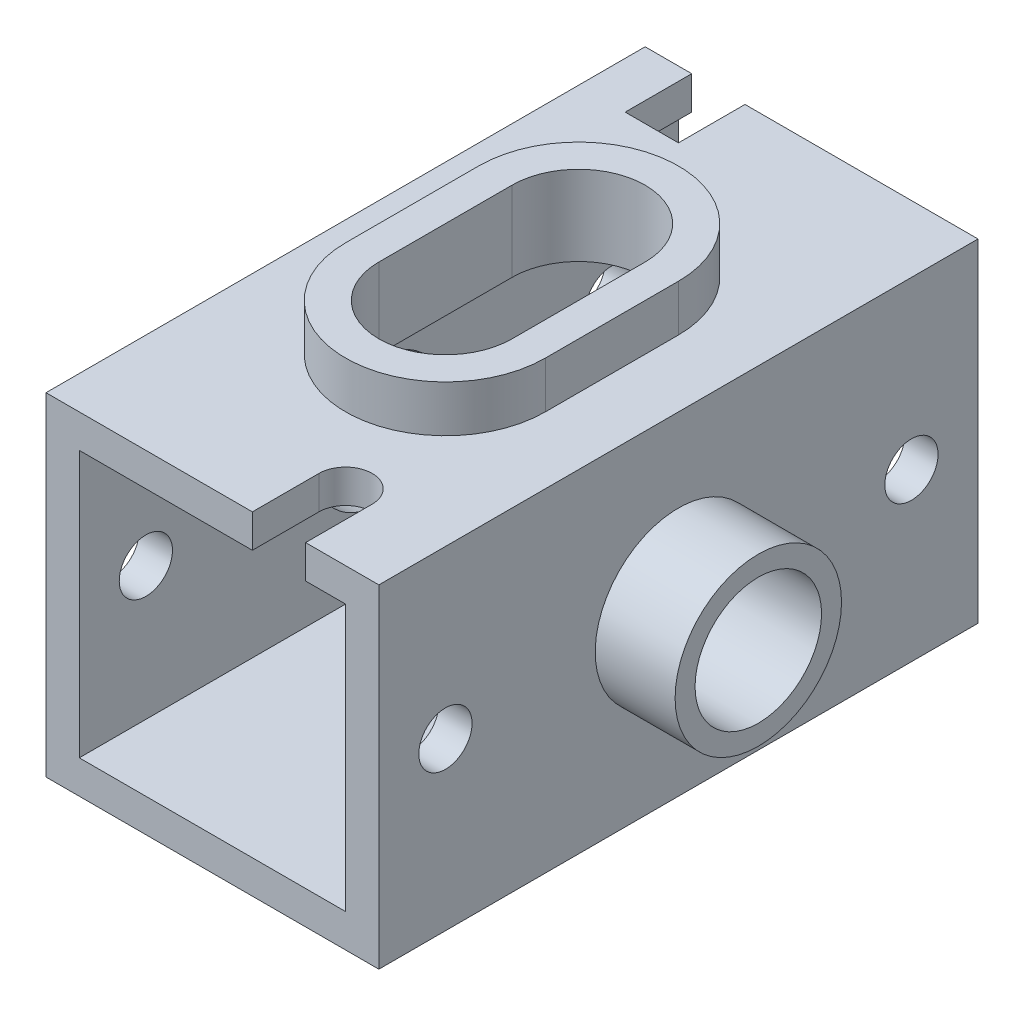
ISO-10303-21;
HEADER;
FILE_DESCRIPTION(('STEP AP214'),'2;1');
FILE_NAME('part.step','',(''),(''),'','','');
FILE_SCHEMA(('AUTOMOTIVE_DESIGN { 1 0 10303 214 1 1 1 1 }'));
ENDSEC;
DATA;
#1=APPLICATION_CONTEXT('core data for automotive mechanical design processes');
#2=APPLICATION_PROTOCOL_DEFINITION('international standard','automotive_design',2000,#1);
#3=PRODUCT_CONTEXT('',#1,'mechanical');
#4=PRODUCT('Part','Part','',(#3));
#5=PRODUCT_RELATED_PRODUCT_CATEGORY('part','',(#4));
#6=PRODUCT_DEFINITION_FORMATION('','',#4);
#7=PRODUCT_DEFINITION_CONTEXT('part definition',#1,'design');
#8=PRODUCT_DEFINITION('design','',#6,#7);
#9=PRODUCT_DEFINITION_SHAPE('','',#8);
#10=(LENGTH_UNIT() NAMED_UNIT(*) SI_UNIT(.MILLI.,.METRE.));
#11=(NAMED_UNIT(*) PLANE_ANGLE_UNIT() SI_UNIT($,.RADIAN.));
#12=(NAMED_UNIT(*) SI_UNIT($,.STERADIAN.) SOLID_ANGLE_UNIT());
#13=UNCERTAINTY_MEASURE_WITH_UNIT(LENGTH_MEASURE(1.E-05),#10,'distance_accuracy_value','');
#14=(GEOMETRIC_REPRESENTATION_CONTEXT(3) GLOBAL_UNCERTAINTY_ASSIGNED_CONTEXT((#13)) GLOBAL_UNIT_ASSIGNED_CONTEXT((#10,
#11,#12)) REPRESENTATION_CONTEXT('',''));
#15=CARTESIAN_POINT('',(0.,0.,0.));
#16=DIRECTION('',(0.,0.,1.));
#17=DIRECTION('',(1.,0.,0.));
#18=AXIS2_PLACEMENT_3D('',#15,#16,#17);
#19=CARTESIAN_POINT('',(-25.,25.,90.));
#20=DIRECTION('',(0.,-1.,0.));
#21=DIRECTION('',(0.,0.,-1.));
#22=AXIS2_PLACEMENT_3D('',#19,#20,#21);
#23=PLANE('',#22);
#24=DIRECTION('',(-1.,0.,0.));
#25=VECTOR('',#24,1.);
#26=CARTESIAN_POINT('',(-25.,25.,90.));
#27=LINE('',#26,#25);
#28=CARTESIAN_POINT('',(5.99999999999999,25.,90.));
#29=VERTEX_POINT('',#28);
#30=CARTESIAN_POINT('',(-25.,25.,90.));
#31=VERTEX_POINT('',#30);
#32=EDGE_CURVE('E400',#29,#31,#27,.T.);
#33=ORIENTED_EDGE('',*,*,#32,.F.);
#34=DIRECTION('',(0.,0.,1.));
#35=VECTOR('',#34,1.);
#36=CARTESIAN_POINT('',(5.99999999999999,25.,80.));
#37=LINE('',#36,#35);
#38=CARTESIAN_POINT('',(5.99999999999999,25.,80.));
#39=VERTEX_POINT('',#38);
#40=EDGE_CURVE('E314',#39,#29,#37,.T.);
#41=ORIENTED_EDGE('',*,*,#40,.F.);
#42=CARTESIAN_POINT('',(9.99999999999999,25.,80.));
#43=DIRECTION('',(0.,1.,0.));
#44=DIRECTION('',(0.,0.,1.));
#45=AXIS2_PLACEMENT_3D('',#42,#43,#44);
#46=CIRCLE('',#45,4.);
#47=CARTESIAN_POINT('',(14.,25.,80.));
#48=VERTEX_POINT('',#47);
#49=EDGE_CURVE('E323',#48,#39,#46,.T.);
#50=ORIENTED_EDGE('',*,*,#49,.F.);
#51=DIRECTION('',(0.,0.,-1.));
#52=VECTOR('',#51,1.);
#53=CARTESIAN_POINT('',(14.,25.,90.));
#54=LINE('',#53,#52);
#55=CARTESIAN_POINT('',(14.,25.,90.));
#56=VERTEX_POINT('',#55);
#57=EDGE_CURVE('E325',#56,#48,#54,.T.);
#58=ORIENTED_EDGE('',*,*,#57,.F.);
#59=CARTESIAN_POINT('',(25.,25.,90.));
#60=VERTEX_POINT('',#59);
#61=EDGE_CURVE('E405',#60,#56,#27,.T.);
#62=ORIENTED_EDGE('',*,*,#61,.F.);
#63=DIRECTION('',(0.,0.,-1.));
#64=VECTOR('',#63,1.);
#65=CARTESIAN_POINT('',(25.,25.,90.));
#66=LINE('',#65,#64);
#67=CARTESIAN_POINT('',(25.,25.,0.));
#68=VERTEX_POINT('',#67);
#69=EDGE_CURVE('E233',#60,#68,#66,.T.);
#70=ORIENTED_EDGE('',*,*,#69,.T.);
#71=DIRECTION('',(-1.,0.,0.));
#72=VECTOR('',#71,1.);
#73=CARTESIAN_POINT('',(-25.,25.,0.));
#74=LINE('',#73,#72);
#75=CARTESIAN_POINT('',(-10.,25.,0.));
#76=VERTEX_POINT('',#75);
#77=EDGE_CURVE('E411',#68,#76,#74,.T.);
#78=ORIENTED_EDGE('',*,*,#77,.T.);
#79=DIRECTION('',(0.,0.,-1.));
#80=VECTOR('',#79,1.);
#81=CARTESIAN_POINT('',(-10.,25.,0.));
#82=LINE('',#81,#80);
#83=CARTESIAN_POINT('',(-10.,25.,10.));
#84=VERTEX_POINT('',#83);
#85=EDGE_CURVE('E344',#84,#76,#82,.T.);
#86=ORIENTED_EDGE('',*,*,#85,.F.);
#87=DIRECTION('',(1.,0.,0.));
#88=VECTOR('',#87,1.);
#89=CARTESIAN_POINT('',(-18.,25.,10.));
#90=LINE('',#89,#88);
#91=CARTESIAN_POINT('',(-18.,25.,10.));
#92=VERTEX_POINT('',#91);
#93=EDGE_CURVE('E352',#92,#84,#90,.T.);
#94=ORIENTED_EDGE('',*,*,#93,.F.);
#95=DIRECTION('',(0.,0.,1.));
#96=VECTOR('',#95,1.);
#97=CARTESIAN_POINT('',(-18.,25.,0.));
#98=LINE('',#97,#96);
#99=CARTESIAN_POINT('',(-18.,25.,0.));
#100=VERTEX_POINT('',#99);
#101=EDGE_CURVE('E309',#100,#92,#98,.T.);
#102=ORIENTED_EDGE('',*,*,#101,.F.);
#103=CARTESIAN_POINT('',(-25.,25.,0.));
#104=VERTEX_POINT('',#103);
#105=EDGE_CURVE('E415',#100,#104,#74,.T.);
#106=ORIENTED_EDGE('',*,*,#105,.T.);
#107=DIRECTION('',(0.,0.,-1.));
#108=VECTOR('',#107,1.);
#109=CARTESIAN_POINT('',(-25.,25.,90.));
#110=LINE('',#109,#108);
#111=EDGE_CURVE('E425',#31,#104,#110,.T.);
#112=ORIENTED_EDGE('',*,*,#111,.F.);
#113=EDGE_LOOP('',(#33,#41,#50,#58,#62,#70,#78,#86,#94,#102,#106,#112));
#114=FACE_BOUND('',#113,.T.);
#115=CARTESIAN_POINT('',(0.,25.,35.));
#116=DIRECTION('',(0.,1.,0.));
#117=DIRECTION('',(0.,0.,1.));
#118=AXIS2_PLACEMENT_3D('',#115,#116,#117);
#119=CIRCLE('',#118,15.);
#120=CARTESIAN_POINT('',(15.,25.,35.));
#121=VERTEX_POINT('',#120);
#122=CARTESIAN_POINT('',(-15.,25.,35.));
#123=VERTEX_POINT('',#122);
#124=EDGE_CURVE('E77',#121,#123,#119,.T.);
#125=ORIENTED_EDGE('',*,*,#124,.F.);
#126=DIRECTION('',(0.,0.,-1.));
#127=VECTOR('',#126,1.);
#128=CARTESIAN_POINT('',(15.,25.,35.));
#129=LINE('',#128,#127);
#130=CARTESIAN_POINT('',(15.,25.,55.));
#131=VERTEX_POINT('',#130);
#132=EDGE_CURVE('E284',#131,#121,#129,.T.);
#133=ORIENTED_EDGE('',*,*,#132,.F.);
#134=CARTESIAN_POINT('',(0.,25.,55.));
#135=DIRECTION('',(0.,1.,0.));
#136=DIRECTION('',(0.,0.,1.));
#137=AXIS2_PLACEMENT_3D('',#134,#135,#136);
#138=CIRCLE('',#137,15.);
#139=CARTESIAN_POINT('',(-15.,25.,55.));
#140=VERTEX_POINT('',#139);
#141=EDGE_CURVE('E294',#140,#131,#138,.T.);
#142=ORIENTED_EDGE('',*,*,#141,.F.);
#143=DIRECTION('',(0.,0.,1.));
#144=VECTOR('',#143,1.);
#145=CARTESIAN_POINT('',(-15.,25.,35.));
#146=LINE('',#145,#144);
#147=EDGE_CURVE('E292',#123,#140,#146,.T.);
#148=ORIENTED_EDGE('',*,*,#147,.F.);
#149=EDGE_LOOP('',(#125,#133,#142,#148));
#150=FACE_BOUND('',#149,.T.);
#151=ADVANCED_FACE('F51',(#114,#150),#23,.F.);
#152=CARTESIAN_POINT('',(0.,0.,90.));
#153=DIRECTION('',(0.,0.,1.));
#154=DIRECTION('',(1.,0.,0.));
#155=AXIS2_PLACEMENT_3D('',#152,#153,#154);
#156=PLANE('',#155);
#157=DIRECTION('',(0.,1.,0.));
#158=VECTOR('',#157,1.);
#159=CARTESIAN_POINT('',(5.99999999999999,20.,90.));
#160=LINE('',#159,#158);
#161=CARTESIAN_POINT('',(5.99999999999999,20.,90.));
#162=VERTEX_POINT('',#161);
#163=EDGE_CURVE('E327',#162,#29,#160,.T.);
#164=ORIENTED_EDGE('',*,*,#163,.T.);
#165=ORIENTED_EDGE('',*,*,#32,.T.);
#166=DIRECTION('',(0.,-1.,0.));
#167=VECTOR('',#166,1.);
#168=CARTESIAN_POINT('',(-25.,25.,90.));
#169=LINE('',#168,#167);
#170=CARTESIAN_POINT('',(-25.,-25.,90.));
#171=VERTEX_POINT('',#170);
#172=EDGE_CURVE('E403',#31,#171,#169,.T.);
#173=ORIENTED_EDGE('',*,*,#172,.T.);
#174=DIRECTION('',(1.,0.,0.));
#175=VECTOR('',#174,1.);
#176=CARTESIAN_POINT('',(-25.,-25.,90.));
#177=LINE('',#176,#175);
#178=CARTESIAN_POINT('',(25.,-25.,90.));
#179=VERTEX_POINT('',#178);
#180=EDGE_CURVE('E410',#171,#179,#177,.T.);
#181=ORIENTED_EDGE('',*,*,#180,.T.);
#182=DIRECTION('',(0.,1.,0.));
#183=VECTOR('',#182,1.);
#184=CARTESIAN_POINT('',(25.,25.,90.));
#185=LINE('',#184,#183);
#186=EDGE_CURVE('E397',#179,#60,#185,.T.);
#187=ORIENTED_EDGE('',*,*,#186,.T.);
#188=ORIENTED_EDGE('',*,*,#61,.T.);
#189=DIRECTION('',(0.,1.,0.));
#190=VECTOR('',#189,1.);
#191=CARTESIAN_POINT('',(14.,20.,90.));
#192=LINE('',#191,#190);
#193=CARTESIAN_POINT('',(14.,20.,90.));
#194=VERTEX_POINT('',#193);
#195=EDGE_CURVE('E322',#194,#56,#192,.T.);
#196=ORIENTED_EDGE('',*,*,#195,.F.);
#197=DIRECTION('',(-1.,0.,0.));
#198=VECTOR('',#197,1.);
#199=CARTESIAN_POINT('',(-20.,20.,90.));
#200=LINE('',#199,#198);
#201=CARTESIAN_POINT('',(20.,20.,90.));
#202=VERTEX_POINT('',#201);
#203=EDGE_CURVE('E361',#202,#194,#200,.T.);
#204=ORIENTED_EDGE('',*,*,#203,.F.);
#205=DIRECTION('',(0.,1.,0.));
#206=VECTOR('',#205,1.);
#207=CARTESIAN_POINT('',(20.,20.,90.));
#208=LINE('',#207,#206);
#209=CARTESIAN_POINT('',(20.,-20.,90.));
#210=VERTEX_POINT('',#209);
#211=EDGE_CURVE('E375',#210,#202,#208,.T.);
#212=ORIENTED_EDGE('',*,*,#211,.F.);
#213=DIRECTION('',(1.,0.,0.));
#214=VECTOR('',#213,1.);
#215=CARTESIAN_POINT('',(-20.,-20.,90.));
#216=LINE('',#215,#214);
#217=CARTESIAN_POINT('',(-20.,-20.,90.));
#218=VERTEX_POINT('',#217);
#219=EDGE_CURVE('E367',#218,#210,#216,.T.);
#220=ORIENTED_EDGE('',*,*,#219,.F.);
#221=DIRECTION('',(0.,-1.,0.));
#222=VECTOR('',#221,1.);
#223=CARTESIAN_POINT('',(-20.,20.,90.));
#224=LINE('',#223,#222);
#225=CARTESIAN_POINT('',(-20.,20.,90.));
#226=VERTEX_POINT('',#225);
#227=EDGE_CURVE('E366',#226,#218,#224,.T.);
#228=ORIENTED_EDGE('',*,*,#227,.F.);
#229=EDGE_CURVE('E370',#162,#226,#200,.T.);
#230=ORIENTED_EDGE('',*,*,#229,.F.);
#231=EDGE_LOOP('',(#164,#165,#173,#181,#187,#188,#196,#204,#212,#220,#228,#230));
#232=FACE_BOUND('',#231,.T.);
#233=ADVANCED_FACE('F453',(#232),#156,.T.);
#234=CARTESIAN_POINT('',(0.,0.,0.));
#235=DIRECTION('',(0.,0.,1.));
#236=DIRECTION('',(1.,0.,0.));
#237=AXIS2_PLACEMENT_3D('',#234,#235,#236);
#238=PLANE('',#237);
#239=ORIENTED_EDGE('',*,*,#105,.F.);
#240=DIRECTION('',(0.,1.,0.));
#241=VECTOR('',#240,1.);
#242=CARTESIAN_POINT('',(-18.,20.,0.));
#243=LINE('',#242,#241);
#244=CARTESIAN_POINT('',(-18.,20.,0.));
#245=VERTEX_POINT('',#244);
#246=EDGE_CURVE('E328',#245,#100,#243,.T.);
#247=ORIENTED_EDGE('',*,*,#246,.F.);
#248=DIRECTION('',(-1.,0.,0.));
#249=VECTOR('',#248,1.);
#250=CARTESIAN_POINT('',(-20.,20.,0.));
#251=LINE('',#250,#249);
#252=CARTESIAN_POINT('',(-20.,20.,0.));
#253=VERTEX_POINT('',#252);
#254=EDGE_CURVE('E334',#245,#253,#251,.T.);
#255=ORIENTED_EDGE('',*,*,#254,.T.);
#256=DIRECTION('',(0.,-1.,0.));
#257=VECTOR('',#256,1.);
#258=CARTESIAN_POINT('',(-20.,20.,0.));
#259=LINE('',#258,#257);
#260=CARTESIAN_POINT('',(-20.,-20.,0.));
#261=VERTEX_POINT('',#260);
#262=EDGE_CURVE('E377',#253,#261,#259,.T.);
#263=ORIENTED_EDGE('',*,*,#262,.T.);
#264=DIRECTION('',(1.,0.,0.));
#265=VECTOR('',#264,1.);
#266=CARTESIAN_POINT('',(-20.,-20.,0.));
#267=LINE('',#266,#265);
#268=CARTESIAN_POINT('',(20.,-20.,0.));
#269=VERTEX_POINT('',#268);
#270=EDGE_CURVE('E382',#261,#269,#267,.T.);
#271=ORIENTED_EDGE('',*,*,#270,.T.);
#272=DIRECTION('',(0.,1.,0.));
#273=VECTOR('',#272,1.);
#274=CARTESIAN_POINT('',(20.,20.,0.));
#275=LINE('',#274,#273);
#276=CARTESIAN_POINT('',(20.,20.,0.));
#277=VERTEX_POINT('',#276);
#278=EDGE_CURVE('E381',#269,#277,#275,.T.);
#279=ORIENTED_EDGE('',*,*,#278,.T.);
#280=CARTESIAN_POINT('',(-10.,20.,0.));
#281=VERTEX_POINT('',#280);
#282=EDGE_CURVE('E374',#277,#281,#251,.T.);
#283=ORIENTED_EDGE('',*,*,#282,.T.);
#284=DIRECTION('',(0.,1.,0.));
#285=VECTOR('',#284,1.);
#286=CARTESIAN_POINT('',(-10.,20.,0.));
#287=LINE('',#286,#285);
#288=EDGE_CURVE('E357',#281,#76,#287,.T.);
#289=ORIENTED_EDGE('',*,*,#288,.T.);
#290=ORIENTED_EDGE('',*,*,#77,.F.);
#291=DIRECTION('',(0.,1.,0.));
#292=VECTOR('',#291,1.);
#293=CARTESIAN_POINT('',(25.,25.,0.));
#294=LINE('',#293,#292);
#295=CARTESIAN_POINT('',(25.,-25.,0.));
#296=VERTEX_POINT('',#295);
#297=EDGE_CURVE('E396',#296,#68,#294,.T.);
#298=ORIENTED_EDGE('',*,*,#297,.F.);
#299=DIRECTION('',(1.,0.,0.));
#300=VECTOR('',#299,1.);
#301=CARTESIAN_POINT('',(-25.,-25.,0.));
#302=LINE('',#301,#300);
#303=CARTESIAN_POINT('',(-25.,-25.,0.));
#304=VERTEX_POINT('',#303);
#305=EDGE_CURVE('E402',#304,#296,#302,.T.);
#306=ORIENTED_EDGE('',*,*,#305,.F.);
#307=DIRECTION('',(0.,-1.,0.));
#308=VECTOR('',#307,1.);
#309=CARTESIAN_POINT('',(-25.,25.,0.));
#310=LINE('',#309,#308);
#311=EDGE_CURVE('E416',#104,#304,#310,.T.);
#312=ORIENTED_EDGE('',*,*,#311,.F.);
#313=EDGE_LOOP('',(#239,#247,#255,#263,#271,#279,#283,#289,#290,#298,#306,#312));
#314=FACE_BOUND('',#313,.T.);
#315=ADVANCED_FACE('F457',(#314),#238,.F.);
#316=CARTESIAN_POINT('',(25.,25.,90.));
#317=DIRECTION('',(-1.,0.,0.));
#318=DIRECTION('',(0.,-1.,0.));
#319=AXIS2_PLACEMENT_3D('',#316,#317,#318);
#320=PLANE('',#319);
#321=CARTESIAN_POINT('',(25.,0.,80.));
#322=DIRECTION('',(1.,0.,0.));
#323=DIRECTION('',(0.,1.,0.));
#324=AXIS2_PLACEMENT_3D('',#321,#322,#323);
#325=CIRCLE('',#324,4.00000000000001);
#326=CARTESIAN_POINT('',(25.,4.00000000000001,80.));
#327=VERTEX_POINT('',#326);
#328=EDGE_CURVE('E590',#327,#327,#325,.T.);
#329=ORIENTED_EDGE('',*,*,#328,.F.);
#330=EDGE_LOOP('',(#329));
#331=FACE_BOUND('',#330,.T.);
#332=CARTESIAN_POINT('',(25.,0.,9.99999999999999));
#333=DIRECTION('',(1.,0.,0.));
#334=DIRECTION('',(0.,1.,0.));
#335=AXIS2_PLACEMENT_3D('',#332,#333,#334);
#336=CIRCLE('',#335,4.);
#337=CARTESIAN_POINT('',(25.,4.,9.99999999999999));
#338=VERTEX_POINT('',#337);
#339=EDGE_CURVE('E260',#338,#338,#336,.T.);
#340=ORIENTED_EDGE('',*,*,#339,.F.);
#341=EDGE_LOOP('',(#340));
#342=FACE_BOUND('',#341,.T.);
#343=CARTESIAN_POINT('',(25.,0.,45.));
#344=DIRECTION('',(-1.,0.,0.));
#345=DIRECTION('',(0.,-1.,0.));
#346=AXIS2_PLACEMENT_3D('',#343,#344,#345);
#347=CIRCLE('',#346,12.5);
#348=CARTESIAN_POINT('',(25.,-12.5,45.));
#349=VERTEX_POINT('',#348);
#350=EDGE_CURVE('E12',#349,#349,#347,.F.);
#351=ORIENTED_EDGE('',*,*,#350,.F.);
#352=EDGE_LOOP('',(#351));
#353=FACE_BOUND('',#352,.T.);
#354=ORIENTED_EDGE('',*,*,#297,.T.);
#355=ORIENTED_EDGE('',*,*,#69,.F.);
#356=ORIENTED_EDGE('',*,*,#186,.F.);
#357=DIRECTION('',(0.,0.,-1.));
#358=VECTOR('',#357,1.);
#359=CARTESIAN_POINT('',(25.,-25.,90.));
#360=LINE('',#359,#358);
#361=EDGE_CURVE('E406',#179,#296,#360,.T.);
#362=ORIENTED_EDGE('',*,*,#361,.T.);
#363=EDGE_LOOP('',(#354,#355,#356,#362));
#364=FACE_BOUND('',#363,.T.);
#365=ADVANCED_FACE('F52',(#331,#342,#353,#364),#320,.F.);
#366=CARTESIAN_POINT('',(-25.,25.,90.));
#367=DIRECTION('',(1.,0.,0.));
#368=DIRECTION('',(0.,1.,0.));
#369=AXIS2_PLACEMENT_3D('',#366,#367,#368);
#370=PLANE('',#369);
#371=CARTESIAN_POINT('',(-25.,0.,45.));
#372=DIRECTION('',(1.,0.,0.));
#373=DIRECTION('',(0.,1.,0.));
#374=AXIS2_PLACEMENT_3D('',#371,#372,#373);
#375=CIRCLE('',#374,12.5);
#376=CARTESIAN_POINT('',(-25.,12.5,45.));
#377=VERTEX_POINT('',#376);
#378=EDGE_CURVE('E580',#377,#377,#375,.T.);
#379=ORIENTED_EDGE('',*,*,#378,.T.);
#380=EDGE_LOOP('',(#379));
#381=FACE_BOUND('',#380,.T.);
#382=CARTESIAN_POINT('',(-25.,0.,80.));
#383=DIRECTION('',(1.,0.,0.));
#384=DIRECTION('',(0.,1.,0.));
#385=AXIS2_PLACEMENT_3D('',#382,#383,#384);
#386=CIRCLE('',#385,4.00000000000001);
#387=CARTESIAN_POINT('',(-25.,4.,80.));
#388=VERTEX_POINT('',#387);
#389=EDGE_CURVE('E242',#388,#388,#386,.T.);
#390=ORIENTED_EDGE('',*,*,#389,.T.);
#391=EDGE_LOOP('',(#390));
#392=FACE_BOUND('',#391,.T.);
#393=CARTESIAN_POINT('',(-25.,0.,9.99999999999999));
#394=DIRECTION('',(1.,0.,0.));
#395=DIRECTION('',(0.,1.,0.));
#396=AXIS2_PLACEMENT_3D('',#393,#394,#395);
#397=CIRCLE('',#396,4.);
#398=CARTESIAN_POINT('',(-25.,4.,9.99999999999999));
#399=VERTEX_POINT('',#398);
#400=EDGE_CURVE('E578',#399,#399,#397,.T.);
#401=ORIENTED_EDGE('',*,*,#400,.T.);
#402=EDGE_LOOP('',(#401));
#403=FACE_BOUND('',#402,.T.);
#404=ORIENTED_EDGE('',*,*,#311,.T.);
#405=DIRECTION('',(0.,0.,-1.));
#406=VECTOR('',#405,1.);
#407=CARTESIAN_POINT('',(-25.,-25.,90.));
#408=LINE('',#407,#406);
#409=EDGE_CURVE('E423',#171,#304,#408,.T.);
#410=ORIENTED_EDGE('',*,*,#409,.F.);
#411=ORIENTED_EDGE('',*,*,#172,.F.);
#412=ORIENTED_EDGE('',*,*,#111,.T.);
#413=EDGE_LOOP('',(#404,#410,#411,#412));
#414=FACE_BOUND('',#413,.T.);
#415=ADVANCED_FACE('F465',(#381,#392,#403,#414),#370,.F.);
#416=CARTESIAN_POINT('',(-25.,-25.,90.));
#417=DIRECTION('',(0.,1.,0.));
#418=DIRECTION('',(0.,0.,1.));
#419=AXIS2_PLACEMENT_3D('',#416,#417,#418);
#420=PLANE('',#419);
#421=ORIENTED_EDGE('',*,*,#305,.T.);
#422=ORIENTED_EDGE('',*,*,#361,.F.);
#423=ORIENTED_EDGE('',*,*,#180,.F.);
#424=ORIENTED_EDGE('',*,*,#409,.T.);
#425=EDGE_LOOP('',(#421,#422,#423,#424));
#426=FACE_BOUND('',#425,.T.);
#427=ADVANCED_FACE('F466',(#426),#420,.F.);
#428=CARTESIAN_POINT('',(-20.,20.,90.));
#429=DIRECTION('',(0.,-1.,0.));
#430=DIRECTION('',(0.,0.,-1.));
#431=AXIS2_PLACEMENT_3D('',#428,#429,#430);
#432=PLANE('',#431);
#433=DIRECTION('',(0.,0.,-1.));
#434=VECTOR('',#433,1.);
#435=CARTESIAN_POINT('',(-9.99999999999999,20.,90.));
#436=LINE('',#435,#434);
#437=CARTESIAN_POINT('',(-10.,20.,55.));
#438=VERTEX_POINT('',#437);
#439=CARTESIAN_POINT('',(-10.,20.,35.));
#440=VERTEX_POINT('',#439);
#441=EDGE_CURVE('E58',#438,#440,#436,.T.);
#442=ORIENTED_EDGE('',*,*,#441,.F.);
#443=CARTESIAN_POINT('',(0.,20.,55.));
#444=DIRECTION('',(0.,-1.,0.));
#445=DIRECTION('',(0.,0.,-1.));
#446=AXIS2_PLACEMENT_3D('',#443,#444,#445);
#447=CIRCLE('',#446,10.);
#448=CARTESIAN_POINT('',(10.,20.,55.));
#449=VERTEX_POINT('',#448);
#450=EDGE_CURVE('E228',#449,#438,#447,.T.);
#451=ORIENTED_EDGE('',*,*,#450,.F.);
#452=DIRECTION('',(0.,0.,-1.));
#453=VECTOR('',#452,1.);
#454=CARTESIAN_POINT('',(10.,20.,90.));
#455=LINE('',#454,#453);
#456=CARTESIAN_POINT('',(10.,20.,35.));
#457=VERTEX_POINT('',#456);
#458=EDGE_CURVE('E229',#449,#457,#455,.T.);
#459=ORIENTED_EDGE('',*,*,#458,.T.);
#460=CARTESIAN_POINT('',(0.,20.,35.));
#461=DIRECTION('',(0.,-1.,0.));
#462=DIRECTION('',(0.,0.,-1.));
#463=AXIS2_PLACEMENT_3D('',#460,#461,#462);
#464=CIRCLE('',#463,10.);
#465=EDGE_CURVE('E236',#440,#457,#464,.T.);
#466=ORIENTED_EDGE('',*,*,#465,.F.);
#467=EDGE_LOOP('',(#442,#451,#459,#466));
#468=FACE_BOUND('',#467,.T.);
#469=DIRECTION('',(0.,0.,1.));
#470=VECTOR('',#469,1.);
#471=CARTESIAN_POINT('',(5.99999999999999,20.,80.));
#472=LINE('',#471,#470);
#473=CARTESIAN_POINT('',(5.99999999999999,20.,80.));
#474=VERTEX_POINT('',#473);
#475=EDGE_CURVE('E319',#474,#162,#472,.T.);
#476=ORIENTED_EDGE('',*,*,#475,.T.);
#477=ORIENTED_EDGE('',*,*,#229,.T.);
#478=DIRECTION('',(0.,0.,-1.));
#479=VECTOR('',#478,1.);
#480=CARTESIAN_POINT('',(-20.,20.,90.));
#481=LINE('',#480,#479);
#482=EDGE_CURVE('E391',#226,#253,#481,.T.);
#483=ORIENTED_EDGE('',*,*,#482,.T.);
#484=ORIENTED_EDGE('',*,*,#254,.F.);
#485=DIRECTION('',(0.,0.,1.));
#486=VECTOR('',#485,1.);
#487=CARTESIAN_POINT('',(-18.,20.,0.));
#488=LINE('',#487,#486);
#489=CARTESIAN_POINT('',(-18.,20.,10.));
#490=VERTEX_POINT('',#489);
#491=EDGE_CURVE('E339',#245,#490,#488,.T.);
#492=ORIENTED_EDGE('',*,*,#491,.T.);
#493=DIRECTION('',(1.,0.,0.));
#494=VECTOR('',#493,1.);
#495=CARTESIAN_POINT('',(-18.,20.,10.));
#496=LINE('',#495,#494);
#497=CARTESIAN_POINT('',(-10.,20.,9.99999999999999));
#498=VERTEX_POINT('',#497);
#499=EDGE_CURVE('E345',#490,#498,#496,.T.);
#500=ORIENTED_EDGE('',*,*,#499,.T.);
#501=DIRECTION('',(0.,0.,-1.));
#502=VECTOR('',#501,1.);
#503=CARTESIAN_POINT('',(-10.,20.,0.));
#504=LINE('',#503,#502);
#505=EDGE_CURVE('E348',#498,#281,#504,.T.);
#506=ORIENTED_EDGE('',*,*,#505,.T.);
#507=ORIENTED_EDGE('',*,*,#282,.F.);
#508=DIRECTION('',(0.,0.,-1.));
#509=VECTOR('',#508,1.);
#510=CARTESIAN_POINT('',(20.,20.,90.));
#511=LINE('',#510,#509);
#512=EDGE_CURVE('E372',#202,#277,#511,.T.);
#513=ORIENTED_EDGE('',*,*,#512,.F.);
#514=ORIENTED_EDGE('',*,*,#203,.T.);
#515=DIRECTION('',(0.,0.,-1.));
#516=VECTOR('',#515,1.);
#517=CARTESIAN_POINT('',(14.,20.,90.));
#518=LINE('',#517,#516);
#519=CARTESIAN_POINT('',(14.,20.,80.));
#520=VERTEX_POINT('',#519);
#521=EDGE_CURVE('E311',#194,#520,#518,.T.);
#522=ORIENTED_EDGE('',*,*,#521,.T.);
#523=CARTESIAN_POINT('',(9.99999999999999,20.,80.));
#524=DIRECTION('',(0.,1.,0.));
#525=DIRECTION('',(0.,0.,1.));
#526=AXIS2_PLACEMENT_3D('',#523,#524,#525);
#527=CIRCLE('',#526,4.);
#528=EDGE_CURVE('E313',#520,#474,#527,.T.);
#529=ORIENTED_EDGE('',*,*,#528,.T.);
#530=EDGE_LOOP('',(#476,#477,#483,#484,#492,#500,#506,#507,#513,#514,#522,#529));
#531=FACE_BOUND('',#530,.T.);
#532=ADVANCED_FACE('F231',(#468,#531),#432,.T.);
#533=CARTESIAN_POINT('',(-20.,20.,90.));
#534=DIRECTION('',(1.,0.,0.));
#535=DIRECTION('',(0.,1.,0.));
#536=AXIS2_PLACEMENT_3D('',#533,#534,#535);
#537=PLANE('',#536);
#538=CARTESIAN_POINT('',(-20.,0.,80.));
#539=DIRECTION('',(1.,0.,0.));
#540=DIRECTION('',(0.,1.,0.));
#541=AXIS2_PLACEMENT_3D('',#538,#539,#540);
#542=CIRCLE('',#541,4.00000000000001);
#543=CARTESIAN_POINT('',(-20.,4.,80.));
#544=VERTEX_POINT('',#543);
#545=EDGE_CURVE('E258',#544,#544,#542,.T.);
#546=ORIENTED_EDGE('',*,*,#545,.F.);
#547=EDGE_LOOP('',(#546));
#548=FACE_BOUND('',#547,.T.);
#549=CARTESIAN_POINT('',(-20.,0.,9.99999999999999));
#550=DIRECTION('',(1.,0.,0.));
#551=DIRECTION('',(0.,1.,0.));
#552=AXIS2_PLACEMENT_3D('',#549,#550,#551);
#553=CIRCLE('',#552,4.);
#554=CARTESIAN_POINT('',(-20.,4.,9.99999999999999));
#555=VERTEX_POINT('',#554);
#556=EDGE_CURVE('E250',#555,#555,#553,.T.);
#557=ORIENTED_EDGE('',*,*,#556,.F.);
#558=EDGE_LOOP('',(#557));
#559=FACE_BOUND('',#558,.T.);
#560=CARTESIAN_POINT('',(-20.,0.,45.));
#561=DIRECTION('',(1.,0.,0.));
#562=DIRECTION('',(0.,1.,0.));
#563=AXIS2_PLACEMENT_3D('',#560,#561,#562);
#564=CIRCLE('',#563,9.49999999999999);
#565=CARTESIAN_POINT('',(-20.,9.49999999999999,45.));
#566=VERTEX_POINT('',#565);
#567=EDGE_CURVE('E243',#566,#566,#564,.T.);
#568=ORIENTED_EDGE('',*,*,#567,.F.);
#569=EDGE_LOOP('',(#568));
#570=FACE_BOUND('',#569,.T.);
#571=ORIENTED_EDGE('',*,*,#262,.F.);
#572=ORIENTED_EDGE('',*,*,#482,.F.);
#573=ORIENTED_EDGE('',*,*,#227,.T.);
#574=DIRECTION('',(0.,0.,-1.));
#575=VECTOR('',#574,1.);
#576=CARTESIAN_POINT('',(-20.,-20.,90.));
#577=LINE('',#576,#575);
#578=EDGE_CURVE('E393',#218,#261,#577,.T.);
#579=ORIENTED_EDGE('',*,*,#578,.T.);
#580=EDGE_LOOP('',(#571,#572,#573,#579));
#581=FACE_BOUND('',#580,.T.);
#582=ADVANCED_FACE('F476',(#548,#559,#570,#581),#537,.T.);
#583=CARTESIAN_POINT('',(-20.,-20.,90.));
#584=DIRECTION('',(0.,1.,0.));
#585=DIRECTION('',(-1.,0.,0.));
#586=AXIS2_PLACEMENT_3D('',#583,#584,#585);
#587=PLANE('',#586);
#588=ORIENTED_EDGE('',*,*,#270,.F.);
#589=ORIENTED_EDGE('',*,*,#578,.F.);
#590=ORIENTED_EDGE('',*,*,#219,.T.);
#591=DIRECTION('',(0.,0.,-1.));
#592=VECTOR('',#591,1.);
#593=CARTESIAN_POINT('',(20.,-20.,90.));
#594=LINE('',#593,#592);
#595=EDGE_CURVE('E386',#210,#269,#594,.T.);
#596=ORIENTED_EDGE('',*,*,#595,.T.);
#597=EDGE_LOOP('',(#588,#589,#590,#596));
#598=FACE_BOUND('',#597,.T.);
#599=ADVANCED_FACE('F481',(#598),#587,.T.);
#600=CARTESIAN_POINT('',(20.,20.,90.));
#601=DIRECTION('',(-1.,0.,0.));
#602=DIRECTION('',(0.,-1.,0.));
#603=AXIS2_PLACEMENT_3D('',#600,#601,#602);
#604=PLANE('',#603);
#605=CARTESIAN_POINT('',(20.,0.,80.));
#606=DIRECTION('',(-1.,0.,0.));
#607=DIRECTION('',(0.,-1.,0.));
#608=AXIS2_PLACEMENT_3D('',#605,#606,#607);
#609=CIRCLE('',#608,4.00000000000001);
#610=CARTESIAN_POINT('',(20.,-4.,80.));
#611=VERTEX_POINT('',#610);
#612=EDGE_CURVE('E54',#611,#611,#609,.T.);
#613=ORIENTED_EDGE('',*,*,#612,.F.);
#614=EDGE_LOOP('',(#613));
#615=FACE_BOUND('',#614,.T.);
#616=CARTESIAN_POINT('',(20.,0.,9.99999999999999));
#617=DIRECTION('',(-1.,0.,0.));
#618=DIRECTION('',(0.,-1.,0.));
#619=AXIS2_PLACEMENT_3D('',#616,#617,#618);
#620=CIRCLE('',#619,4.);
#621=CARTESIAN_POINT('',(20.,-4.,9.99999999999999));
#622=VERTEX_POINT('',#621);
#623=EDGE_CURVE('E244',#622,#622,#620,.T.);
#624=ORIENTED_EDGE('',*,*,#623,.F.);
#625=EDGE_LOOP('',(#624));
#626=FACE_BOUND('',#625,.T.);
#627=CARTESIAN_POINT('',(20.,0.,45.));
#628=DIRECTION('',(-1.,0.,0.));
#629=DIRECTION('',(0.,-1.,0.));
#630=AXIS2_PLACEMENT_3D('',#627,#628,#629);
#631=CIRCLE('',#630,9.49999999999999);
#632=CARTESIAN_POINT('',(20.,-9.49999999999999,45.));
#633=VERTEX_POINT('',#632);
#634=EDGE_CURVE('E241',#633,#633,#631,.T.);
#635=ORIENTED_EDGE('',*,*,#634,.F.);
#636=EDGE_LOOP('',(#635));
#637=FACE_BOUND('',#636,.T.);
#638=ORIENTED_EDGE('',*,*,#278,.F.);
#639=ORIENTED_EDGE('',*,*,#595,.F.);
#640=ORIENTED_EDGE('',*,*,#211,.T.);
#641=ORIENTED_EDGE('',*,*,#512,.T.);
#642=EDGE_LOOP('',(#638,#639,#640,#641));
#643=FACE_BOUND('',#642,.T.);
#644=ADVANCED_FACE('F485',(#615,#626,#637,#643),#604,.T.);
#645=CARTESIAN_POINT('',(-18.,20.,0.));
#646=DIRECTION('',(-1.,0.,0.));
#647=DIRECTION('',(0.,0.,1.));
#648=AXIS2_PLACEMENT_3D('',#645,#646,#647);
#649=PLANE('',#648);
#650=ORIENTED_EDGE('',*,*,#101,.T.);
#651=DIRECTION('',(0.,1.,0.));
#652=VECTOR('',#651,1.);
#653=CARTESIAN_POINT('',(-18.,20.,10.));
#654=LINE('',#653,#652);
#655=EDGE_CURVE('E349',#490,#92,#654,.T.);
#656=ORIENTED_EDGE('',*,*,#655,.F.);
#657=ORIENTED_EDGE('',*,*,#491,.F.);
#658=ORIENTED_EDGE('',*,*,#246,.T.);
#659=EDGE_LOOP('',(#650,#656,#657,#658));
#660=FACE_BOUND('',#659,.T.);
#661=ADVANCED_FACE('F490',(#660),#649,.F.);
#662=CARTESIAN_POINT('',(-10.,20.,0.));
#663=DIRECTION('',(1.,0.,0.));
#664=DIRECTION('',(0.,0.,-1.));
#665=AXIS2_PLACEMENT_3D('',#662,#663,#664);
#666=PLANE('',#665);
#667=ORIENTED_EDGE('',*,*,#85,.T.);
#668=ORIENTED_EDGE('',*,*,#288,.F.);
#669=ORIENTED_EDGE('',*,*,#505,.F.);
#670=DIRECTION('',(0.,1.,0.));
#671=VECTOR('',#670,1.);
#672=CARTESIAN_POINT('',(-10.,20.,10.));
#673=LINE('',#672,#671);
#674=EDGE_CURVE('E359',#498,#84,#673,.T.);
#675=ORIENTED_EDGE('',*,*,#674,.T.);
#676=EDGE_LOOP('',(#667,#668,#669,#675));
#677=FACE_BOUND('',#676,.T.);
#678=ADVANCED_FACE('F491',(#677),#666,.F.);
#679=CARTESIAN_POINT('',(-18.,20.,10.));
#680=DIRECTION('',(0.,0.,1.));
#681=DIRECTION('',(1.,0.,0.));
#682=AXIS2_PLACEMENT_3D('',#679,#680,#681);
#683=PLANE('',#682);
#684=ORIENTED_EDGE('',*,*,#93,.T.);
#685=ORIENTED_EDGE('',*,*,#674,.F.);
#686=ORIENTED_EDGE('',*,*,#499,.F.);
#687=ORIENTED_EDGE('',*,*,#655,.T.);
#688=EDGE_LOOP('',(#684,#685,#686,#687));
#689=FACE_BOUND('',#688,.T.);
#690=ADVANCED_FACE('F492',(#689),#683,.F.);
#691=CARTESIAN_POINT('',(5.99999999999999,20.,80.));
#692=DIRECTION('',(-1.,0.,0.));
#693=DIRECTION('',(0.,0.,1.));
#694=AXIS2_PLACEMENT_3D('',#691,#692,#693);
#695=PLANE('',#694);
#696=ORIENTED_EDGE('',*,*,#40,.T.);
#697=ORIENTED_EDGE('',*,*,#163,.F.);
#698=ORIENTED_EDGE('',*,*,#475,.F.);
#699=DIRECTION('',(0.,1.,0.));
#700=VECTOR('',#699,1.);
#701=CARTESIAN_POINT('',(5.99999999999999,20.,80.));
#702=LINE('',#701,#700);
#703=EDGE_CURVE('E333',#474,#39,#702,.T.);
#704=ORIENTED_EDGE('',*,*,#703,.T.);
#705=EDGE_LOOP('',(#696,#697,#698,#704));
#706=FACE_BOUND('',#705,.T.);
#707=ADVANCED_FACE('F498',(#706),#695,.F.);
#708=CARTESIAN_POINT('',(9.99999999999999,20.,80.));
#709=DIRECTION('',(0.,1.,0.));
#710=DIRECTION('',(0.,0.,1.));
#711=AXIS2_PLACEMENT_3D('',#708,#709,#710);
#712=CYLINDRICAL_SURFACE('',#711,4.);
#713=ORIENTED_EDGE('',*,*,#49,.T.);
#714=ORIENTED_EDGE('',*,*,#703,.F.);
#715=ORIENTED_EDGE('',*,*,#528,.F.);
#716=DIRECTION('',(0.,1.,0.));
#717=VECTOR('',#716,1.);
#718=CARTESIAN_POINT('',(14.,20.,80.));
#719=LINE('',#718,#717);
#720=EDGE_CURVE('E337',#520,#48,#719,.T.);
#721=ORIENTED_EDGE('',*,*,#720,.T.);
#722=EDGE_LOOP('',(#713,#714,#715,#721));
#723=FACE_BOUND('',#722,.T.);
#724=ADVANCED_FACE('F448',(#723),#712,.F.);
#725=CARTESIAN_POINT('',(14.,20.,90.));
#726=DIRECTION('',(1.,0.,0.));
#727=DIRECTION('',(0.,0.,-1.));
#728=AXIS2_PLACEMENT_3D('',#725,#726,#727);
#729=PLANE('',#728);
#730=ORIENTED_EDGE('',*,*,#57,.T.);
#731=ORIENTED_EDGE('',*,*,#720,.F.);
#732=ORIENTED_EDGE('',*,*,#521,.F.);
#733=ORIENTED_EDGE('',*,*,#195,.T.);
#734=EDGE_LOOP('',(#730,#731,#732,#733));
#735=FACE_BOUND('',#734,.T.);
#736=ADVANCED_FACE('F437',(#735),#729,.F.);
#737=CARTESIAN_POINT('',(0.,32.,35.));
#738=DIRECTION('',(0.,1.,0.));
#739=DIRECTION('',(0.,0.,1.));
#740=AXIS2_PLACEMENT_3D('',#737,#738,#739);
#741=PLANE('',#740);
#742=CARTESIAN_POINT('',(0.,32.,35.));
#743=DIRECTION('',(0.,1.,0.));
#744=DIRECTION('',(0.,0.,1.));
#745=AXIS2_PLACEMENT_3D('',#742,#743,#744);
#746=CIRCLE('',#745,15.);
#747=CARTESIAN_POINT('',(15.,32.,35.));
#748=VERTEX_POINT('',#747);
#749=CARTESIAN_POINT('',(-15.,32.,35.));
#750=VERTEX_POINT('',#749);
#751=EDGE_CURVE('E278',#748,#750,#746,.T.);
#752=ORIENTED_EDGE('',*,*,#751,.T.);
#753=DIRECTION('',(0.,0.,1.));
#754=VECTOR('',#753,1.);
#755=CARTESIAN_POINT('',(-15.,32.,35.));
#756=LINE('',#755,#754);
#757=CARTESIAN_POINT('',(-15.,32.,55.));
#758=VERTEX_POINT('',#757);
#759=EDGE_CURVE('E281',#750,#758,#756,.T.);
#760=ORIENTED_EDGE('',*,*,#759,.T.);
#761=CARTESIAN_POINT('',(0.,32.,55.));
#762=DIRECTION('',(0.,1.,0.));
#763=DIRECTION('',(0.,0.,1.));
#764=AXIS2_PLACEMENT_3D('',#761,#762,#763);
#765=CIRCLE('',#764,15.);
#766=CARTESIAN_POINT('',(15.,32.,55.));
#767=VERTEX_POINT('',#766);
#768=EDGE_CURVE('E286',#758,#767,#765,.T.);
#769=ORIENTED_EDGE('',*,*,#768,.T.);
#770=DIRECTION('',(0.,0.,-1.));
#771=VECTOR('',#770,1.);
#772=CARTESIAN_POINT('',(15.,32.,35.));
#773=LINE('',#772,#771);
#774=EDGE_CURVE('E289',#767,#748,#773,.T.);
#775=ORIENTED_EDGE('',*,*,#774,.T.);
#776=EDGE_LOOP('',(#752,#760,#769,#775));
#777=FACE_BOUND('',#776,.T.);
#778=DIRECTION('',(0.,0.,1.));
#779=VECTOR('',#778,1.);
#780=CARTESIAN_POINT('',(-10.,32.,35.));
#781=LINE('',#780,#779);
#782=CARTESIAN_POINT('',(-10.,32.,35.));
#783=VERTEX_POINT('',#782);
#784=CARTESIAN_POINT('',(-10.,32.,55.));
#785=VERTEX_POINT('',#784);
#786=EDGE_CURVE('E221',#783,#785,#781,.T.);
#787=ORIENTED_EDGE('',*,*,#786,.F.);
#788=CARTESIAN_POINT('',(0.,32.,35.));
#789=DIRECTION('',(0.,1.,0.));
#790=DIRECTION('',(0.,0.,1.));
#791=AXIS2_PLACEMENT_3D('',#788,#789,#790);
#792=CIRCLE('',#791,10.);
#793=CARTESIAN_POINT('',(10.,32.,35.));
#794=VERTEX_POINT('',#793);
#795=EDGE_CURVE('E268',#794,#783,#792,.T.);
#796=ORIENTED_EDGE('',*,*,#795,.F.);
#797=DIRECTION('',(0.,0.,-1.));
#798=VECTOR('',#797,1.);
#799=CARTESIAN_POINT('',(10.,32.,35.));
#800=LINE('',#799,#798);
#801=CARTESIAN_POINT('',(10.,32.,55.));
#802=VERTEX_POINT('',#801);
#803=EDGE_CURVE('E274',#802,#794,#800,.T.);
#804=ORIENTED_EDGE('',*,*,#803,.F.);
#805=CARTESIAN_POINT('',(0.,32.,55.));
#806=DIRECTION('',(0.,1.,0.));
#807=DIRECTION('',(0.,0.,1.));
#808=AXIS2_PLACEMENT_3D('',#805,#806,#807);
#809=CIRCLE('',#808,10.);
#810=EDGE_CURVE('E275',#785,#802,#809,.T.);
#811=ORIENTED_EDGE('',*,*,#810,.F.);
#812=EDGE_LOOP('',(#787,#796,#804,#811));
#813=FACE_BOUND('',#812,.T.);
#814=ADVANCED_FACE('F436',(#777,#813),#741,.T.);
#815=CARTESIAN_POINT('',(0.,32.,35.));
#816=DIRECTION('',(0.,-1.,0.));
#817=DIRECTION('',(0.,0.,-1.));
#818=AXIS2_PLACEMENT_3D('',#815,#816,#817);
#819=CYLINDRICAL_SURFACE('',#818,15.);
#820=ORIENTED_EDGE('',*,*,#124,.T.);
#821=DIRECTION('',(0.,-1.,0.));
#822=VECTOR('',#821,1.);
#823=CARTESIAN_POINT('',(-15.,32.,35.));
#824=LINE('',#823,#822);
#825=EDGE_CURVE('E310',#750,#123,#824,.T.);
#826=ORIENTED_EDGE('',*,*,#825,.F.);
#827=ORIENTED_EDGE('',*,*,#751,.F.);
#828=DIRECTION('',(0.,-1.,0.));
#829=VECTOR('',#828,1.);
#830=CARTESIAN_POINT('',(15.,32.,35.));
#831=LINE('',#830,#829);
#832=EDGE_CURVE('E290',#748,#121,#831,.T.);
#833=ORIENTED_EDGE('',*,*,#832,.T.);
#834=EDGE_LOOP('',(#820,#826,#827,#833));
#835=FACE_BOUND('',#834,.T.);
#836=ADVANCED_FACE('F438',(#835),#819,.T.);
#837=CARTESIAN_POINT('',(-15.,32.,35.));
#838=DIRECTION('',(1.,0.,0.));
#839=DIRECTION('',(0.,0.,-1.));
#840=AXIS2_PLACEMENT_3D('',#837,#838,#839);
#841=PLANE('',#840);
#842=ORIENTED_EDGE('',*,*,#147,.T.);
#843=DIRECTION('',(0.,-1.,0.));
#844=VECTOR('',#843,1.);
#845=CARTESIAN_POINT('',(-15.,32.,55.));
#846=LINE('',#845,#844);
#847=EDGE_CURVE('E302',#758,#140,#846,.T.);
#848=ORIENTED_EDGE('',*,*,#847,.F.);
#849=ORIENTED_EDGE('',*,*,#759,.F.);
#850=ORIENTED_EDGE('',*,*,#825,.T.);
#851=EDGE_LOOP('',(#842,#848,#849,#850));
#852=FACE_BOUND('',#851,.T.);
#853=ADVANCED_FACE('F447',(#852),#841,.F.);
#854=CARTESIAN_POINT('',(0.,32.,55.));
#855=DIRECTION('',(0.,-1.,0.));
#856=DIRECTION('',(0.,0.,-1.));
#857=AXIS2_PLACEMENT_3D('',#854,#855,#856);
#858=CYLINDRICAL_SURFACE('',#857,15.);
#859=ORIENTED_EDGE('',*,*,#141,.T.);
#860=DIRECTION('',(0.,-1.,0.));
#861=VECTOR('',#860,1.);
#862=CARTESIAN_POINT('',(15.,32.,55.));
#863=LINE('',#862,#861);
#864=EDGE_CURVE('E301',#767,#131,#863,.T.);
#865=ORIENTED_EDGE('',*,*,#864,.F.);
#866=ORIENTED_EDGE('',*,*,#768,.F.);
#867=ORIENTED_EDGE('',*,*,#847,.T.);
#868=EDGE_LOOP('',(#859,#865,#866,#867));
#869=FACE_BOUND('',#868,.T.);
#870=ADVANCED_FACE('F512',(#869),#858,.T.);
#871=CARTESIAN_POINT('',(15.,32.,35.));
#872=DIRECTION('',(-1.,0.,0.));
#873=DIRECTION('',(0.,0.,1.));
#874=AXIS2_PLACEMENT_3D('',#871,#872,#873);
#875=PLANE('',#874);
#876=ORIENTED_EDGE('',*,*,#132,.T.);
#877=ORIENTED_EDGE('',*,*,#832,.F.);
#878=ORIENTED_EDGE('',*,*,#774,.F.);
#879=ORIENTED_EDGE('',*,*,#864,.T.);
#880=EDGE_LOOP('',(#876,#877,#878,#879));
#881=FACE_BOUND('',#880,.T.);
#882=ADVANCED_FACE('F511',(#881),#875,.F.);
#883=CARTESIAN_POINT('',(0.,32.,35.));
#884=DIRECTION('',(0.,-1.,0.));
#885=DIRECTION('',(0.,0.,-1.));
#886=AXIS2_PLACEMENT_3D('',#883,#884,#885);
#887=CYLINDRICAL_SURFACE('',#886,10.);
#888=DIRECTION('',(0.,-1.,0.));
#889=VECTOR('',#888,1.);
#890=CARTESIAN_POINT('',(-10.,32.,35.));
#891=LINE('',#890,#889);
#892=EDGE_CURVE('E224',#783,#440,#891,.T.);
#893=ORIENTED_EDGE('',*,*,#892,.T.);
#894=ORIENTED_EDGE('',*,*,#465,.T.);
#895=DIRECTION('',(0.,-1.,0.));
#896=VECTOR('',#895,1.);
#897=CARTESIAN_POINT('',(10.,32.,35.));
#898=LINE('',#897,#896);
#899=EDGE_CURVE('E277',#794,#457,#898,.T.);
#900=ORIENTED_EDGE('',*,*,#899,.F.);
#901=ORIENTED_EDGE('',*,*,#795,.T.);
#902=EDGE_LOOP('',(#893,#894,#900,#901));
#903=FACE_BOUND('',#902,.T.);
#904=ADVANCED_FACE('F432',(#903),#887,.F.);
#905=CARTESIAN_POINT('',(-10.,32.,35.));
#906=DIRECTION('',(1.,0.,0.));
#907=DIRECTION('',(0.,0.,-1.));
#908=AXIS2_PLACEMENT_3D('',#905,#906,#907);
#909=PLANE('',#908);
#910=DIRECTION('',(0.,-1.,0.));
#911=VECTOR('',#910,1.);
#912=CARTESIAN_POINT('',(-10.,32.,55.));
#913=LINE('',#912,#911);
#914=EDGE_CURVE('E213',#785,#438,#913,.T.);
#915=ORIENTED_EDGE('',*,*,#914,.T.);
#916=ORIENTED_EDGE('',*,*,#441,.T.);
#917=ORIENTED_EDGE('',*,*,#892,.F.);
#918=ORIENTED_EDGE('',*,*,#786,.T.);
#919=EDGE_LOOP('',(#915,#916,#917,#918));
#920=FACE_BOUND('',#919,.T.);
#921=ADVANCED_FACE('F218',(#920),#909,.T.);
#922=CARTESIAN_POINT('',(0.,32.,55.));
#923=DIRECTION('',(0.,-1.,0.));
#924=DIRECTION('',(0.,0.,-1.));
#925=AXIS2_PLACEMENT_3D('',#922,#923,#924);
#926=CYLINDRICAL_SURFACE('',#925,10.);
#927=DIRECTION('',(0.,-1.,0.));
#928=VECTOR('',#927,1.);
#929=CARTESIAN_POINT('',(10.,32.,55.));
#930=LINE('',#929,#928);
#931=EDGE_CURVE('E66',#802,#449,#930,.T.);
#932=ORIENTED_EDGE('',*,*,#931,.T.);
#933=ORIENTED_EDGE('',*,*,#450,.T.);
#934=ORIENTED_EDGE('',*,*,#914,.F.);
#935=ORIENTED_EDGE('',*,*,#810,.T.);
#936=EDGE_LOOP('',(#932,#933,#934,#935));
#937=FACE_BOUND('',#936,.T.);
#938=ADVANCED_FACE('F227',(#937),#926,.F.);
#939=CARTESIAN_POINT('',(10.,32.,35.));
#940=DIRECTION('',(-1.,0.,0.));
#941=DIRECTION('',(0.,0.,1.));
#942=AXIS2_PLACEMENT_3D('',#939,#940,#941);
#943=PLANE('',#942);
#944=ORIENTED_EDGE('',*,*,#899,.T.);
#945=ORIENTED_EDGE('',*,*,#458,.F.);
#946=ORIENTED_EDGE('',*,*,#931,.F.);
#947=ORIENTED_EDGE('',*,*,#803,.T.);
#948=EDGE_LOOP('',(#944,#945,#946,#947));
#949=FACE_BOUND('',#948,.T.);
#950=ADVANCED_FACE('F429',(#949),#943,.T.);
#951=CARTESIAN_POINT('',(37.,0.,45.));
#952=DIRECTION('',(1.,0.,0.));
#953=DIRECTION('',(0.,1.,0.));
#954=AXIS2_PLACEMENT_3D('',#951,#952,#953);
#955=PLANE('',#954);
#956=CARTESIAN_POINT('',(37.,0.,45.));
#957=DIRECTION('',(1.,0.,0.));
#958=DIRECTION('',(0.,1.,0.));
#959=AXIS2_PLACEMENT_3D('',#956,#957,#958);
#960=CIRCLE('',#959,12.5);
#961=CARTESIAN_POINT('',(37.,12.5,45.));
#962=VERTEX_POINT('',#961);
#963=EDGE_CURVE('E266',#962,#962,#960,.T.);
#964=ORIENTED_EDGE('',*,*,#963,.T.);
#965=EDGE_LOOP('',(#964));
#966=FACE_BOUND('',#965,.T.);
#967=CARTESIAN_POINT('',(37.,0.,45.));
#968=DIRECTION('',(1.,0.,0.));
#969=DIRECTION('',(0.,1.,0.));
#970=AXIS2_PLACEMENT_3D('',#967,#968,#969);
#971=CIRCLE('',#970,9.49999999999999);
#972=CARTESIAN_POINT('',(37.,9.5,45.));
#973=VERTEX_POINT('',#972);
#974=EDGE_CURVE('E261',#973,#973,#971,.T.);
#975=ORIENTED_EDGE('',*,*,#974,.F.);
#976=EDGE_LOOP('',(#975));
#977=FACE_BOUND('',#976,.T.);
#978=ADVANCED_FACE('F540',(#966,#977),#955,.T.);
#979=CARTESIAN_POINT('',(37.,0.,45.));
#980=DIRECTION('',(-1.,0.,0.));
#981=DIRECTION('',(0.,-1.,0.));
#982=AXIS2_PLACEMENT_3D('',#979,#980,#981);
#983=CYLINDRICAL_SURFACE('',#982,12.5);
#984=ORIENTED_EDGE('',*,*,#963,.F.);
#985=EDGE_LOOP('',(#984));
#986=FACE_BOUND('',#985,.T.);
#987=ORIENTED_EDGE('',*,*,#350,.T.);
#988=EDGE_LOOP('',(#987));
#989=FACE_BOUND('',#988,.T.);
#990=ADVANCED_FACE('F539',(#986,#989),#983,.T.);
#991=CARTESIAN_POINT('',(37.,0.,45.));
#992=DIRECTION('',(-1.,0.,0.));
#993=DIRECTION('',(0.,-1.,0.));
#994=AXIS2_PLACEMENT_3D('',#991,#992,#993);
#995=CYLINDRICAL_SURFACE('',#994,9.49999999999999);
#996=ORIENTED_EDGE('',*,*,#974,.T.);
#997=EDGE_LOOP('',(#996));
#998=FACE_BOUND('',#997,.T.);
#999=ORIENTED_EDGE('',*,*,#634,.T.);
#1000=EDGE_LOOP('',(#999));
#1001=FACE_BOUND('',#1000,.T.);
#1002=ADVANCED_FACE('F543',(#998,#1001),#995,.F.);
#1003=CARTESIAN_POINT('',(-25.,0.,9.99999999999999));
#1004=DIRECTION('',(1.,0.,0.));
#1005=DIRECTION('',(0.,1.,0.));
#1006=AXIS2_PLACEMENT_3D('',#1003,#1004,#1005);
#1007=CYLINDRICAL_SURFACE('',#1006,4.);
#1008=ORIENTED_EDGE('',*,*,#623,.T.);
#1009=EDGE_LOOP('',(#1008));
#1010=FACE_BOUND('',#1009,.T.);
#1011=ORIENTED_EDGE('',*,*,#339,.T.);
#1012=EDGE_LOOP('',(#1011));
#1013=FACE_BOUND('',#1012,.T.);
#1014=ADVANCED_FACE('F549',(#1010,#1013),#1007,.F.);
#1015=CARTESIAN_POINT('',(-25.,0.,80.));
#1016=DIRECTION('',(1.,0.,0.));
#1017=DIRECTION('',(0.,1.,0.));
#1018=AXIS2_PLACEMENT_3D('',#1015,#1016,#1017);
#1019=CYLINDRICAL_SURFACE('',#1018,4.00000000000001);
#1020=ORIENTED_EDGE('',*,*,#612,.T.);
#1021=EDGE_LOOP('',(#1020));
#1022=FACE_BOUND('',#1021,.T.);
#1023=ORIENTED_EDGE('',*,*,#328,.T.);
#1024=EDGE_LOOP('',(#1023));
#1025=FACE_BOUND('',#1024,.T.);
#1026=ADVANCED_FACE('F555',(#1022,#1025),#1019,.F.);
#1027=CARTESIAN_POINT('',(-25.,0.,45.));
#1028=DIRECTION('',(1.,0.,0.));
#1029=DIRECTION('',(0.,1.,0.));
#1030=AXIS2_PLACEMENT_3D('',#1027,#1028,#1029);
#1031=CYLINDRICAL_SURFACE('',#1030,9.49999999999999);
#1032=ORIENTED_EDGE('',*,*,#567,.T.);
#1033=EDGE_LOOP('',(#1032));
#1034=FACE_BOUND('',#1033,.T.);
#1035=CARTESIAN_POINT('',(-37.,0.,45.));
#1036=DIRECTION('',(1.,0.,0.));
#1037=DIRECTION('',(0.,1.,0.));
#1038=AXIS2_PLACEMENT_3D('',#1035,#1036,#1037);
#1039=CIRCLE('',#1038,9.49999999999999);
#1040=CARTESIAN_POINT('',(-37.,9.5,45.));
#1041=VERTEX_POINT('',#1040);
#1042=EDGE_CURVE('E572',#1041,#1041,#1039,.T.);
#1043=ORIENTED_EDGE('',*,*,#1042,.F.);
#1044=EDGE_LOOP('',(#1043));
#1045=FACE_BOUND('',#1044,.T.);
#1046=ADVANCED_FACE('F550',(#1034,#1045),#1031,.F.);
#1047=ORIENTED_EDGE('',*,*,#556,.T.);
#1048=EDGE_LOOP('',(#1047));
#1049=FACE_BOUND('',#1048,.T.);
#1050=ORIENTED_EDGE('',*,*,#400,.F.);
#1051=EDGE_LOOP('',(#1050));
#1052=FACE_BOUND('',#1051,.T.);
#1053=ADVANCED_FACE('F551',(#1049,#1052),#1007,.F.);
#1054=ORIENTED_EDGE('',*,*,#545,.T.);
#1055=EDGE_LOOP('',(#1054));
#1056=FACE_BOUND('',#1055,.T.);
#1057=ORIENTED_EDGE('',*,*,#389,.F.);
#1058=EDGE_LOOP('',(#1057));
#1059=FACE_BOUND('',#1058,.T.);
#1060=ADVANCED_FACE('F557',(#1056,#1059),#1019,.F.);
#1061=CARTESIAN_POINT('',(-37.,0.,45.));
#1062=DIRECTION('',(1.,0.,0.));
#1063=DIRECTION('',(0.,1.,0.));
#1064=AXIS2_PLACEMENT_3D('',#1061,#1062,#1063);
#1065=CYLINDRICAL_SURFACE('',#1064,12.5);
#1066=CARTESIAN_POINT('',(-37.,0.,45.));
#1067=DIRECTION('',(1.,0.,0.));
#1068=DIRECTION('',(0.,1.,0.));
#1069=AXIS2_PLACEMENT_3D('',#1066,#1067,#1068);
#1070=CIRCLE('',#1069,12.5);
#1071=CARTESIAN_POINT('',(-37.,12.5,45.));
#1072=VERTEX_POINT('',#1071);
#1073=EDGE_CURVE('E577',#1072,#1072,#1070,.T.);
#1074=ORIENTED_EDGE('',*,*,#1073,.T.);
#1075=EDGE_LOOP('',(#1074));
#1076=FACE_BOUND('',#1075,.T.);
#1077=ORIENTED_EDGE('',*,*,#378,.F.);
#1078=EDGE_LOOP('',(#1077));
#1079=FACE_BOUND('',#1078,.T.);
#1080=ADVANCED_FACE('F561',(#1076,#1079),#1065,.T.);
#1081=CARTESIAN_POINT('',(-37.,0.,45.));
#1082=DIRECTION('',(-1.,0.,0.));
#1083=DIRECTION('',(0.,1.,0.));
#1084=AXIS2_PLACEMENT_3D('',#1081,#1082,#1083);
#1085=PLANE('',#1084);
#1086=ORIENTED_EDGE('',*,*,#1042,.T.);
#1087=EDGE_LOOP('',(#1086));
#1088=FACE_BOUND('',#1087,.T.);
#1089=ORIENTED_EDGE('',*,*,#1073,.F.);
#1090=EDGE_LOOP('',(#1089));
#1091=FACE_BOUND('',#1090,.T.);
#1092=ADVANCED_FACE('F562',(#1088,#1091),#1085,.T.);
#1093=CLOSED_SHELL('',(#151,#233,#315,#365,#415,#427,#532,#582,#599,#644,#661,#678,#690,#707,
#724,#736,#814,#836,#853,#870,#882,#904,#921,#938,#950,#978,#990,#1002,#1014,#1026,#1046,#1053,
#1060,#1080,#1092));
#1094=MANIFOLD_SOLID_BREP('B2',#1093);
#1095=ADVANCED_BREP_SHAPE_REPRESENTATION('',(#18,#1094),#14);
#1096=SHAPE_DEFINITION_REPRESENTATION(#9,#1095);
ENDSEC;
END-ISO-10303-21;
